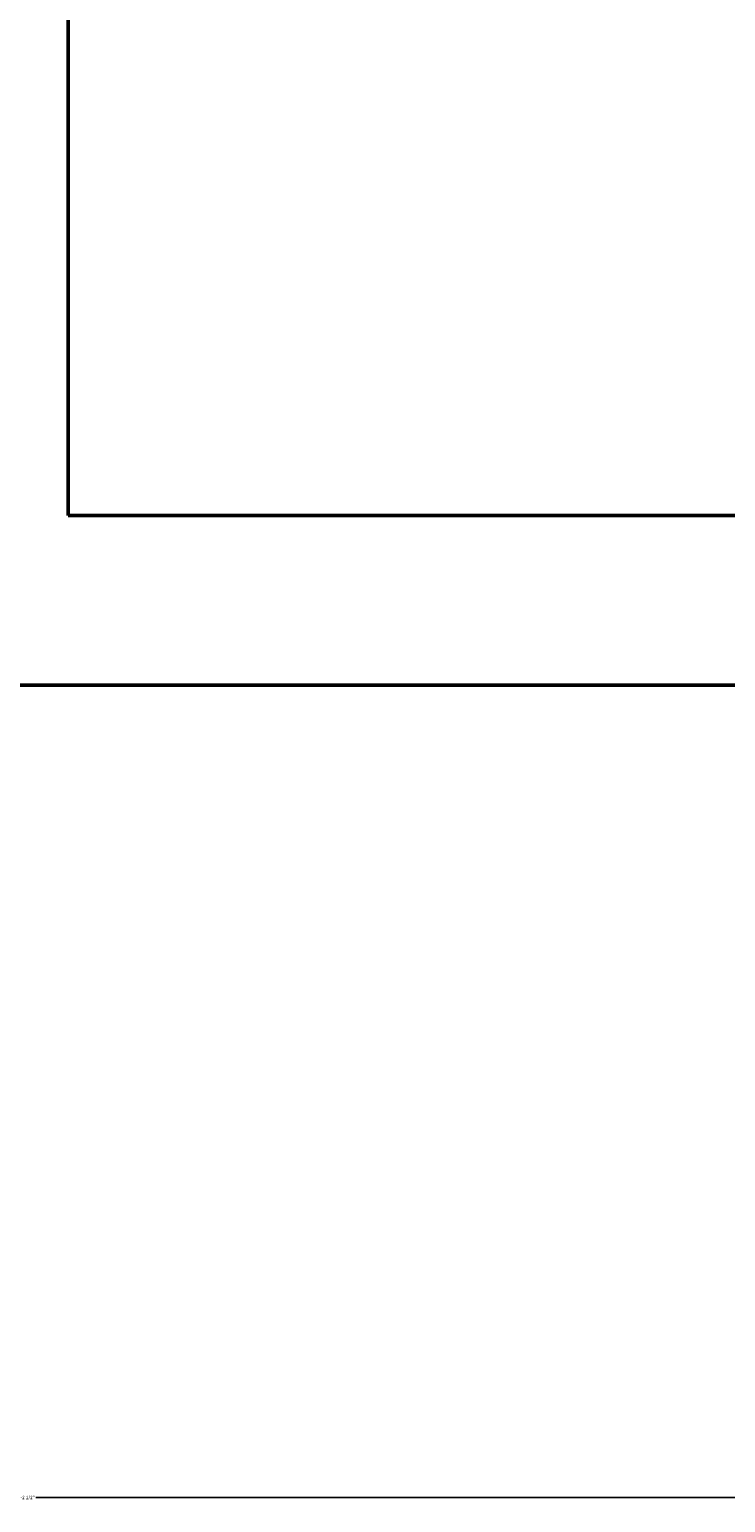
# Model space of a CAD drawing. Units: inches. Extents: x -173 to 545, y -746 to 104.
# Tile 8 of 32: x 263 to 300, y -741 to -663. Entities that reach past the tile are written whole.
import ezdxf

# ---------------------------------------------------------------- set-up
doc = ezdxf.new("R2010")
doc.units = ezdxf.units.IN
doc.header["$MEASUREMENT"] = 0
doc.layers.add('A-ANNO-DIMS', color=2, linetype='Continuous', lineweight=18)
doc.layers.add('A-WALL', color=7, linetype='Continuous', lineweight=50)
doc.styles.get("Standard").update_dxf_attribs({"font": 'arial.ttf'})
doc.dimstyles.get("Standard").update_dxf_attribs({"dimtxt": 0.18, "dimasz": 0.18, "dimexe": 0.18, "dimexo": 0.0625, "dimgap": 0.09, "dimtad": 0, "dimtih": 1, "dimtoh": 1, "dimdec": 0, "dimzin": 0, "dimdsep": 46, "dimlunit": 3, "dimtxsty": 'Standard', "dimcen": 0.09, "dimadec": 0, "dimazin": 0, "dimtfac": 1, "dimtdec": 0, "dimtofl": 0, "dimtmove": 0, "dimatfit": 3, "dimfxl": 1, "dimtolj": 1, "dimtzin": 0, "dimarcsym": 0})

# ---------------------------------------------------------------- blocks, each defined once
blk = doc.blocks.new('*D81')
at = {"layer": 'A-ANNO-DIMS', "color": 0, "lineweight": -2, "transparency": 16777216}
for p, q in [((219.801, -551.924), (219.801, -740.642)), ((306.301, -551.924), (306.301, -740.642)), ((219.981, -740.462), (262.513, -740.462)), ((306.121, -740.462), (263.59, -740.462))]:
    blk.add_line(p, q, dxfattribs=at)
at = {"layer": 'A-ANNO-DIMS', "color": 0, "transparency": 16777216}
for points in [[(219.981, -740.432), (219.981, -740.492), (219.801, -740.462)], [(306.121, -740.432), (306.121, -740.492), (306.301, -740.462)]]:
    blk.add_solid(points, dxfattribs=at)
at = {"layer": 'Defpoints', "color": 0, "transparency": 16777216}
for p in [(219.801, -551.862), (306.301, -551.862), (306.301, -740.462)]:
    blk.add_point(p, dxfattribs=at)
at = {"layer": 'A-ANNO-DIMS', "color": 0, "transparency": 16777216, "insert": (263.051, -740.462), "char_height": 0.18, "attachment_point": 5}
blk.add_mtext('\\A1;7\'-2 1/2"', dxfattribs=at)

msp = doc.modelspace()

# ---------------------------------------------------------------- linework, layer by layer
at = {"layer": 'A-WALL'}
for p, q in [((265.301, -560.862), (265.301, -688.362)), ((265.301, -688.362), (356.301, -688.362)), ((24.301, -697.362), (501.801, -697.362))]:
    msp.add_line(p, q, dxfattribs=at)

# ---------------------------------------------------------------- dimensions: what is measured, and where the dimension line sits
at = {"layer": 'A-ANNO-DIMS'}
dim = msp.add_linear_dim(base=(306.301, -740.462), p1=(219.801, -551.862), p2=(306.301, -551.862), dimstyle='Standard', override={"dimdec": 1, "dimlfac": 1, "dimrnd": 0, "dimzin": 1, "dimdsep": 46, "dimlunit": 4, "dimfrac": 2}, dxfattribs=at)
dim.commit()
dim.dimension.update_dxf_attribs({"geometry": '*D81', "text_midpoint": (263.051, -740.462)})

doc.saveas('drawing.dxf')
